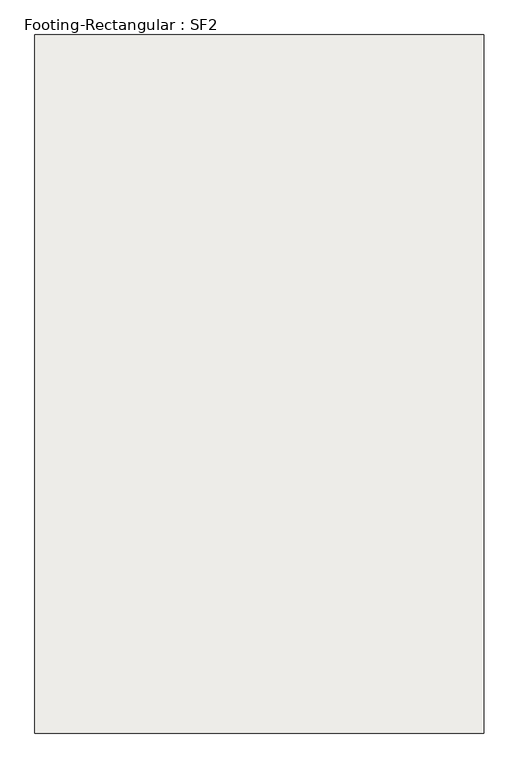
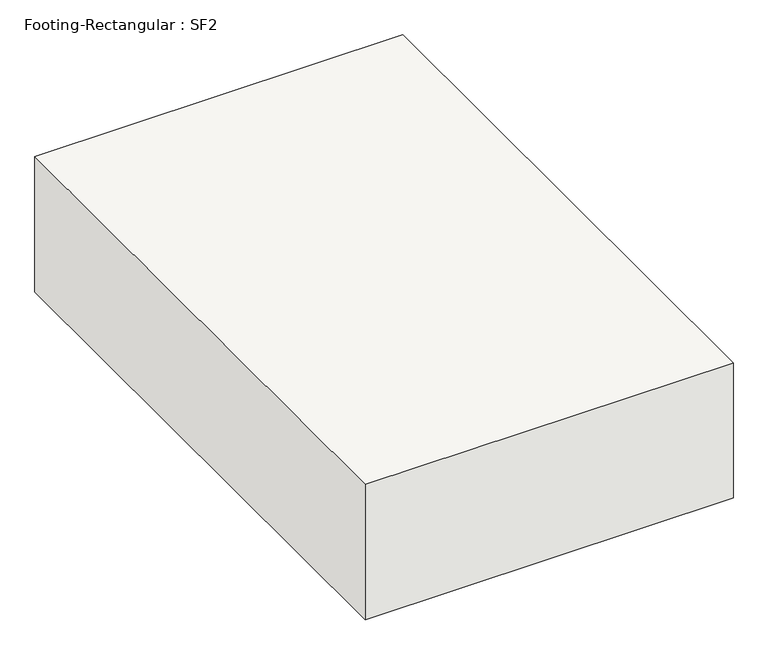
"""IFC4 building model written with IfcOpenShell, lengths in millimetres: slab geometry, Footing-Rectangular : SF2."""

from ifc_helpers import new_model, si_unit, frame, origin, place, context, project, spatial, polyline, outline, extrude, source, transform, mapped, element, save


def footing_rectangular_sf2_5cd490c0(model_context):
    return source(origin(), model_context, "Body", "SweptSolid", [
        extrude(outline(polyline([(685.8, 1066.8), (685.8, -1066.8), (-685.8, -1066.8), (-685.8, 1066.8), (685.8, 1066.8)])), frame((0.0, 0.0, -533.4), z_axis=(0.0, 0.0, 1.0), x_axis=(1.0, 0.0, 0.0)), (0.0, 0.0, 1.0), 533.4),
    ])


if __name__ == "__main__":
    model = new_model("IFC4")
    model_context = context("Model", 3, world=origin())
    ifc_project = project(units=[si_unit("LENGTHUNIT", "METRE", prefix="MILLI")], contexts=[model_context])
    site = spatial("IfcSite", under=ifc_project)
    building = spatial("IfcBuilding", under=site)
    placement = place(None, origin())
    footing_rectangular_sf2_shape = footing_rectangular_sf2_5cd490c0(model_context)
    element("IfcSlab", 1, ObjectType="Footing-Rectangular : SF2", at=placement, inside=building, context=model_context, shape_type="MappedRepresentation", body=[
        mapped(footing_rectangular_sf2_shape, transform((0.0, 0.0, 0.0), x_axis=(1.0, 0.0, 0.0), y_axis=(0.0, 1.0, 0.0), z_axis=(0.0, 0.0, 1.0))),
    ])
    save(model, "model.ifc")

# Revit data of these elements
# Type "Footing-Rectangular : SF2"
#   Width = 1371.6 mm
#   Length = 2133.6 mm
#   Foundation Thickness = 533.4 mm
#   Structural Material [instance default] = Concrete - Cast-in-Place Concrete
#   Assembly Code = ""
# Element 1 (IfcSlab, "Footing-Rectangular : SF2")
#   Materials on its faces: "Concrete - Cast-in-Place Concrete"
# Materials
#   "Concrete - Cast-in-Place Concrete": class "Concrete", colour RGB 192 192 192, transparency 0, Cost = 0
